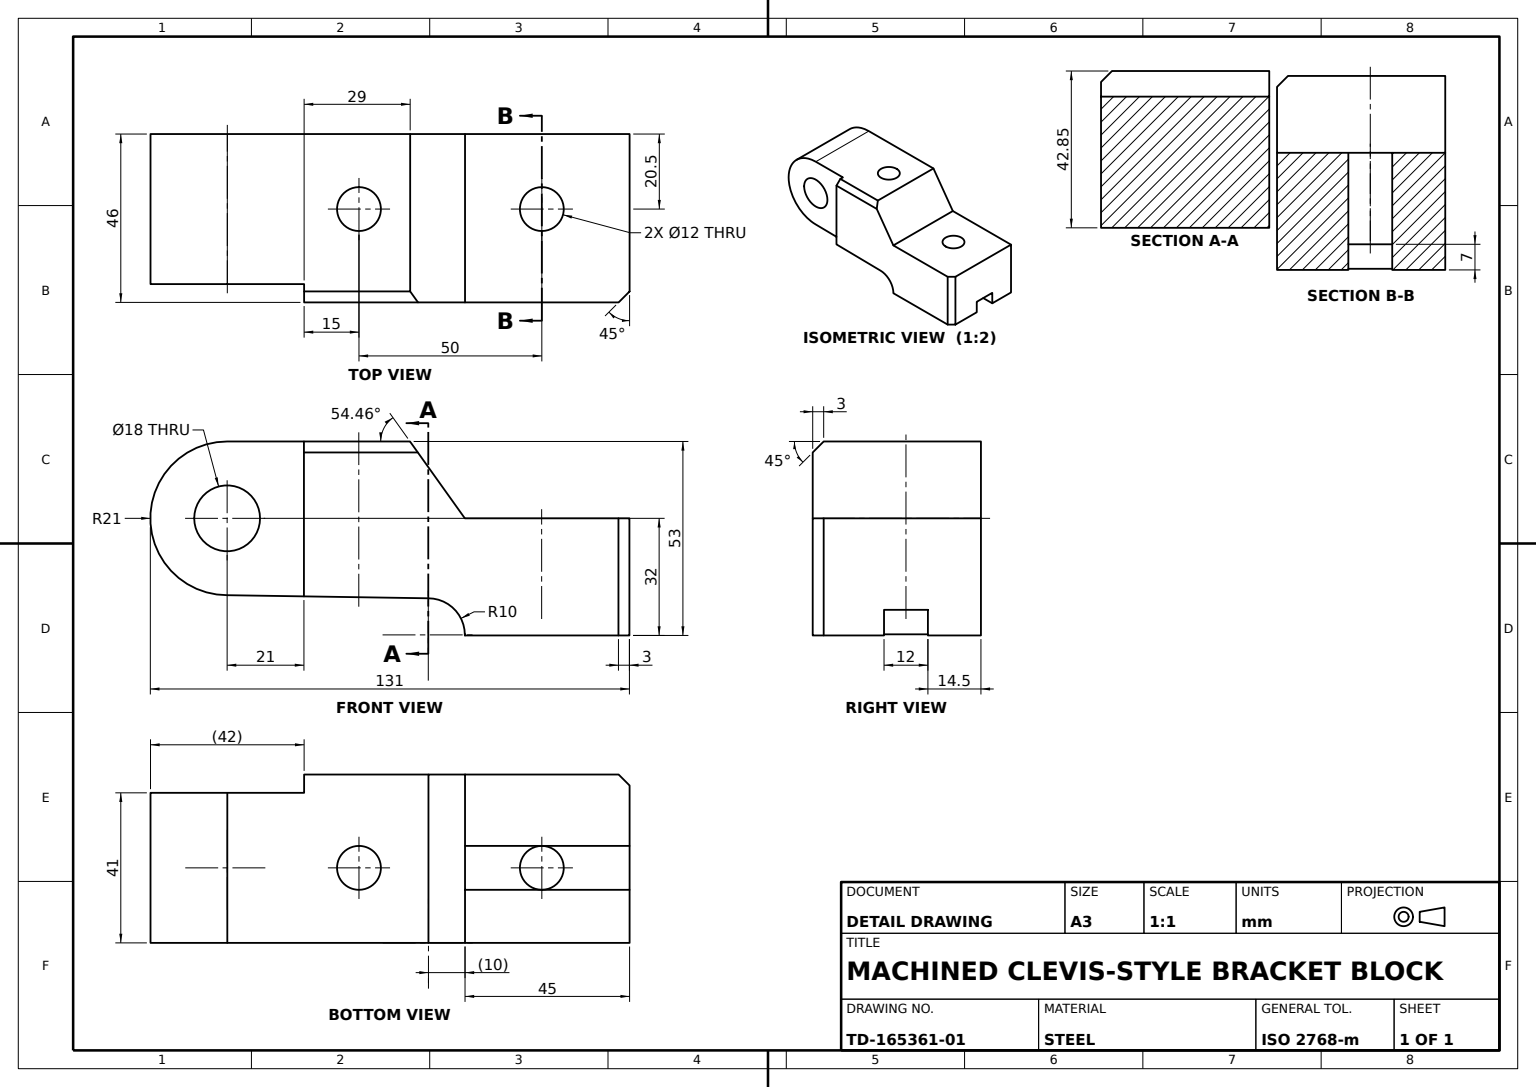
from build123d import *

# Parameters (mm, degrees)
BASE_BLOCK_PROFILE_W       = 45
BASE_BLOCK_PROFILE_H       = 32
BASE_BLOCK_DEPTH           = 41
END_SLOT_PROFILE_W         = 12
END_SLOT_PROFILE_H         = 7
END_SLOT_7X12_DEPTH        = 45
ARM_EXTENSION_DEPTH        = 41
UNDERSIDE_RELIEF_PROFILE_R = 6
UNDERSIDE_RELIEF_CUT_DEPTH = 50
RAISED_START               = 5
RAISED_PAD_DEPTH           = 5
PIVOT_BORE_PROFILE_R       = 9
PIVOT_BORE_18_DEPTH        = 50
PAD_CHAMFER_3X45_A_SIZE    = 3
PAD_CHAMFER_3X45_B_SIZE    = 3


with BuildPart() as part:
    # Base Block Profile → Base Block (new body)
    with BuildSketch(Plane.XY):
        with Locations((22.5, -16)):
            Rectangle(BASE_BLOCK_PROFILE_W, BASE_BLOCK_PROFILE_H)
    extrude(amount=BASE_BLOCK_DEPTH)

    # End Slot Profile → End Slot 7x12 (cut)
    with BuildSketch(Plane(origin=(45, 0, 0), x_dir=(0, 0, -1), z_dir=(1, 0, 0))):
        with Locations((-20.5, -28.5)):
            Rectangle(END_SLOT_PROFILE_W, END_SLOT_PROFILE_H)
    extrude(amount=-END_SLOT_7X12_DEPTH, mode=Mode.SUBTRACT)

    # Arm Extension Profile → Arm Extension (add)
    with BuildSketch(Plane.XY.offset(41)):
        with BuildLine():
            Line((-15, 21), (-65, 21))
            ThreePointArc((-65, 21), (-86, 0), (-65, -21))
            Line((-65, -21), (-9.998816778, -21.84617205))
            ThreePointArc((-9.998816778, -21.84617205), (-9.844988828, -21.847355271), (-9.69119728, -21.850904657))
            ThreePointArc((-9.69119728, -21.850904657), (-2.873570133, -24.829701409), (0, -31.692344099))
            Line((0, -31.692344099), (0, -22))
            Line((0, -22), (0, 0))
            Line((0, 0), (-15, 21))
        make_face()
    extrude(amount=-ARM_EXTENSION_DEPTH)

    # Underside Relief Profile → Underside Relief Cut (cut)
    with BuildSketch(Plane(origin=(0, 21, 0), x_dir=(1, 0, 0), z_dir=(0, 1, 0))):
        with Locations(Location((-29, -20.5, 0), (0, 0, 270))):
            Circle(UNDERSIDE_RELIEF_PROFILE_R)
        with Locations(Location((21, -20.5, 0), (0, 0, 90))):
            Circle(UNDERSIDE_RELIEF_PROFILE_R)
    extrude(amount=-UNDERSIDE_RELIEF_CUT_DEPTH, mode=Mode.SUBTRACT)

    # Raised Pad Profile → Raised Pad (add)
    with BuildSketch(Plane.XY.offset(41).offset(RAISED_START)):
        with BuildLine():
            Line((-44, 21), (-44, 0))
            Line((-44, 0), (-44, -21.323076923))
            Line((-44, -21.323076923), (-9.998816778, -21.84617205))
            ThreePointArc((-9.998816778, -21.84617205), (-2.982346138, -24.720925405), (0, -31.692344099))
            ThreePointArc((0, -31.692344099), (0.001183222, -31.84617205), (0, -32))
            Line((0, -32), (45, -32))
            Line((45, -32), (45, 0))
            Line((45, 0), (0, 0))
            Line((0, 0), (-15, 21))
            Line((-15, 21), (-44, 21))
        make_face()
    extrude(amount=-RAISED_PAD_DEPTH)

    # Pivot Bore Profile → Pivot Bore Ø18 (cut)
    with BuildSketch(Plane.XY.offset(41)):
        with Locations((-65, 0)):
            Circle(PIVOT_BORE_PROFILE_R)
    extrude(amount=-PIVOT_BORE_18_DEPTH, mode=Mode.SUBTRACT)

    # Pad Chamfer 3x45 A
    pad_chamfer_3x45_a_edges = [part.edges().sort_by_distance(p)[0] for p in [
        (-29.5, 21, 46),
    ]]
    chamfer(pad_chamfer_3x45_a_edges, length=PAD_CHAMFER_3X45_A_SIZE)

    # Pad Chamfer 3x45 B
    pad_chamfer_3x45_b_edges = [part.edges().sort_by_distance(p)[0] for p in [
        (45, -16, 46),
    ]]
    chamfer(pad_chamfer_3x45_b_edges, length=PAD_CHAMFER_3X45_B_SIZE)


solid = part.part
